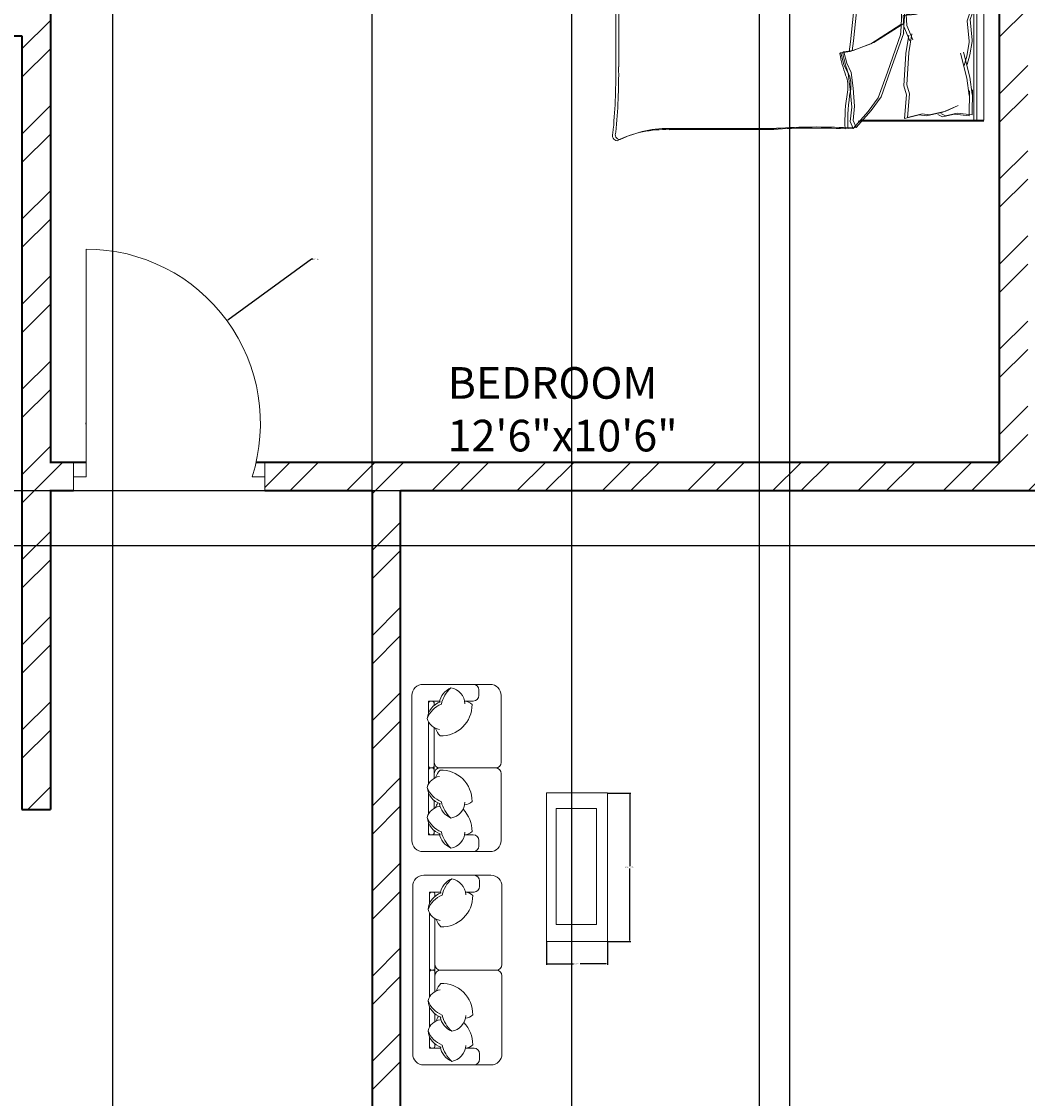
# Model space of a CAD drawing. Units: inches. Extents: x 2064 to 2782, y 1196 to 2299.
# Tile 7 of 11: x 2331 to 2490, y 1963 to 2133. Entities that reach past the tile are written whole.
import ezdxf

# ---------------------------------------------------------------- set-up
doc = ezdxf.new("R2010")
doc.units = ezdxf.units.IN
for name, color, linetype, lineweight in [('A-ANNO-DIMS', 2, 'Continuous', 18), ('A-AREA-IDEN', 7, 'Continuous', 18), ('A-DOOR', 11, 'Continuous', 18), ('A-FURN', 8, 'Continuous', 13), ('A-WALL', 7, 'Continuous', 35), ('A-WALL-PATT', 9, 'Continuous', 13)]:
    doc.layers.add(name, color=color, linetype=linetype, lineweight=lineweight)
doc.styles.get("Standard").update_dxf_attribs({"font": 'arial.ttf'})
doc.dimstyles.get("Standard").update_dxf_attribs({"dimtxt": 0.18, "dimasz": 0.18, "dimexe": 0.18, "dimexo": 0.0625, "dimgap": 0.09, "dimtad": 0, "dimtih": 1, "dimtoh": 1, "dimdec": 4, "dimzin": 0, "dimdsep": 46, "dimtxsty": 'Standard', "dimcen": 0.09, "dimadec": 0, "dimazin": 0, "dimtfac": 1, "dimtdec": 4, "dimtofl": 0, "dimtmove": 0, "dimatfit": 3, "dimfxl": 1, "dimtolj": 1, "dimtzin": 0, "dimarcsym": 0})

# ---------------------------------------------------------------- blocks, each defined once
blk = doc.blocks.new('BED-DOUBLE')
for p, q in [((2.53, 46.14), (2.53, 59.33)), ((2.53, 46.14), (2.53, 59.33)), ((2.53, 59.33), (37.35, 59.33)), ((2.53, 58.22), (37.35, 58.22)), ((2.53, 58.22), (37.35, 58.22)), ((2.7, 45.67), (2.7, 58.87)), ((2.7, 45.67), (2.7, 58.87)), ((17.88, 57.55), (18.93, 57.97)), ((17.88, 57.55), (18.93, 57.97)), ((18.93, 57.97), (19.35, 54.07)), ((18.93, 57.97), (19.35, 54.07)), ((37.35, 59.33), (37.35, 39.95)), ((37.35, 59.33), (37.35, 39.95)), ((37.52, 59.33), (37.52, 58.87)), ((37.52, 58.87), (37.52, 39.48)), ((37.52, 58.87), (37.52, 39.48)), ((2.7, 57.75), (37.52, 57.75)), ((2.7, 57.75), (37.52, 57.75)), ((2.84, 56.9), (5.96, 57.14)), ((2.84, 56.9), (5.96, 57.14)), ((2.84, 56.92), (3.26, 54.6)), ((2.84, 56.92), (3.26, 54.6)), ((3, 56.45), (3.43, 54.14)), ((3, 56.45), (3.43, 54.14)), ((3.01, 56.44), (6.13, 56.68)), ((3.01, 56.44), (6.13, 56.68)), ((5.96, 57.14), (6.04, 57.13)), ((5.96, 57.14), (6.04, 57.13)), ((6.04, 57.13), (8.82, 56.92)), ((6.04, 57.13), (8.82, 56.92)), ((6.13, 56.68), (6.2, 56.66)), ((6.13, 56.68), (6.2, 56.66)), ((6.2, 56.66), (8.99, 56.45)), ((6.2, 56.66), (8.99, 56.45)), ((8.82, 56.92), (12.82, 56.18)), ((8.82, 56.92), (12.82, 56.18)), ((8.99, 56.45), (12.99, 55.72)), ((8.99, 56.45), (12.99, 55.72)), ((10.82, 56.6), (12.3, 57.13)), ((10.82, 56.6), (12.3, 57.13)), ((10.99, 56.14), (12.46, 56.66)), ((10.99, 56.14), (12.46, 56.66)), ((12.3, 57.13), (14.4, 57.66)), ((12.3, 57.13), (14.4, 57.66)), ((12.46, 56.66), (14.57, 57.19)), ((12.46, 56.66), (14.57, 57.19)), ((14.4, 57.66), (14.64, 57.66)), ((14.4, 57.66), (14.64, 57.66)), ((14.57, 57.19), (14.8, 57.19)), ((14.57, 57.19), (14.8, 57.19)), ((14.64, 57.66), (17.88, 57.55)), ((14.64, 57.66), (17.88, 57.55)), ((14.8, 57.19), (18.04, 57.09)), ((14.8, 57.19), (18.04, 57.09)), ((18.04, 57.09), (19.1, 57.51)), ((18.04, 57.09), (19.1, 57.51)), ((19.1, 57.51), (19.52, 53.61)), ((19.1, 57.51), (19.52, 53.61)), ((20.38, 57.52), (20.2, 53.6)), ((20.38, 57.52), (20.21, 53.6)), ((20.55, 57.05), (20.37, 53.14)), ((20.55, 57.05), (20.37, 53.14)), ((21.46, 57.16), (20.38, 57.52)), ((21.46, 57.16), (20.38, 57.52)), ((21.63, 56.7), (20.55, 57.05)), ((21.63, 56.7), (20.55, 57.05)), ((24.69, 57.47), (21.46, 57.16)), ((24.69, 57.47), (21.46, 57.16)), ((24.85, 57.01), (21.63, 56.7)), ((24.85, 57.01), (21.63, 56.7)), ((24.92, 57.49), (24.69, 57.47)), ((24.92, 57.49), (24.69, 57.47)), ((25.09, 57.02), (24.85, 57.01)), ((25.09, 57.02), (24.85, 57.01)), ((27.05, 57.09), (24.92, 57.49)), ((27.05, 57.09), (24.92, 57.49)), ((27.22, 56.63), (25.09, 57.02)), ((27.22, 56.63), (25.09, 57.02)), ((30.54, 57.1), (26.59, 56.11)), ((30.54, 57.1), (26.59, 56.11)), ((30.7, 56.63), (26.75, 55.65)), ((30.7, 56.63), (26.75, 55.65)), ((28.56, 56.66), (27.05, 57.09)), ((28.56, 56.66), (27.05, 57.09)), ((28.73, 56.19), (27.22, 56.63)), ((28.73, 56.19), (27.22, 56.63)), ((33.3, 57.48), (30.54, 57.1)), ((33.3, 57.48), (30.54, 57.1)), ((33.47, 57.02), (30.7, 56.63)), ((33.47, 57.02), (30.7, 56.63)), ((36.51, 57.47), (32.57, 57.54)), ((32.57, 57.54), (33.3, 57.48)), ((36.51, 57.47), (32.57, 57.54)), ((32.57, 57.54), (33.3, 57.48)), ((36.68, 57.01), (32.74, 57.08)), ((32.74, 57.08), (33.47, 57.02)), ((36.67, 57.01), (32.74, 57.08)), ((32.74, 57.08), (33.47, 57.02)), ((36.51, 57.47), (36.23, 55.13)), ((36.51, 57.47), (36.23, 55.13)), ((36.68, 57.01), (36.4, 54.67)), ((36.67, 57.01), (36.4, 54.67)), ((3.26, 54.6), (2.94, 52.71)), ((3.26, 54.6), (2.94, 52.71)), ((3.68, 52.81), (4.42, 54.81)), ((3.68, 52.81), (4.42, 54.81)), ((35.92, 53.32), (35.06, 55.27)), ((35.92, 53.32), (35.06, 55.27)), ((36.09, 52.85), (35.23, 54.8)), ((36.09, 52.85), (35.23, 54.8)), ((36.23, 55.13), (36.67, 53.26)), ((36.23, 55.13), (36.67, 53.26)), ((36.4, 54.67), (36.83, 52.79)), ((36.4, 54.67), (36.83, 52.79)), ((3.43, 54.14), (3.11, 52.24)), ((3.43, 54.14), (3.11, 52.24)), ((3.26, 50.18), (3.68, 52.81)), ((3.26, 50.18), (3.68, 52.81)), ((3.85, 52.34), (4.58, 54.35)), ((3.85, 52.34), (4.58, 54.35)), ((19.35, 54.07), (19.77, 51.76)), ((19.35, 54.07), (19.77, 51.76)), ((19.52, 53.61), (19.94, 51.29)), ((19.52, 53.61), (19.94, 51.29)), ((20.21, 53.6), (19.93, 51.26)), ((20.2, 53.6), (19.93, 51.26)), ((20.37, 53.14), (20.1, 50.8)), ((20.37, 53.14), (20.1, 50.8)), ((36.51, 50.72), (35.92, 53.32)), ((36.51, 50.72), (35.92, 53.32)), ((36.68, 50.25), (36.09, 52.85)), ((36.67, 50.25), (36.09, 52.85)), ((36.67, 53.26), (36.29, 52.5)), ((36.67, 53.26), (36.29, 52.5)), ((2.94, 52.71), (3.36, 51.97)), ((2.94, 52.71), (3.36, 51.97)), ((3.11, 52.24), (3.53, 51.5)), ((3.11, 52.24), (3.53, 51.5)), ((3.43, 49.71), (3.85, 52.34)), ((3.43, 49.71), (3.85, 52.34)), ((19.77, 51.76), (19.77, 50.81)), ((19.77, 51.76), (19.77, 50.81)), ((19.93, 51.26), (19.99, 50.32)), ((19.93, 51.26), (19.99, 50.32)), ((19.94, 51.29), (19.94, 50.34)), ((19.94, 51.29), (19.94, 50.34)), ((36.83, 52.79), (36.46, 52.03)), ((36.83, 52.79), (36.46, 52.03)), ((3.47, 49.02), (3.26, 50.18)), ((3.47, 49.02), (3.26, 50.18)), ((3.64, 48.55), (3.43, 49.71)), ((3.64, 48.55), (3.43, 49.71)), ((19.77, 50.81), (19.35, 49.44)), ((19.77, 50.81), (19.35, 49.44)), ((19.35, 49.44), (19.35, 47.49)), ((19.35, 49.44), (19.35, 47.49)), ((19.94, 50.34), (19.52, 48.97)), ((19.94, 50.34), (19.52, 48.97)), ((19.99, 50.32), (20.49, 48.98)), ((19.99, 50.32), (20.49, 48.98)), ((20.1, 50.8), (20.15, 49.85)), ((20.1, 50.8), (20.15, 49.85)), ((20.15, 49.85), (20.66, 48.51)), ((20.15, 49.85), (20.66, 48.51)), ((36.37, 49.55), (36.51, 50.72)), ((36.37, 49.55), (36.51, 50.72)), ((36.94, 47.26), (36.37, 49.55)), ((36.94, 47.26), (36.37, 49.55)), ((36.54, 49.08), (36.68, 50.25)), ((36.54, 49.08), (36.67, 50.25)), ((3.05, 46.7), (3.47, 49.02)), ((3.05, 46.7), (3.47, 49.02)), ((3.21, 46.24), (3.64, 48.55)), ((3.21, 46.24), (3.64, 48.55)), ((4.65, 47.95), (7.59, 47.46)), ((4.65, 47.95), (7.59, 47.46)), ((17.56, 47.49), (15.27, 48.28)), ((17.56, 47.49), (15.27, 48.28)), ((17.73, 47.02), (15.44, 47.82)), ((17.73, 47.02), (15.44, 47.82)), ((19.52, 48.97), (19.52, 47.02)), ((19.52, 48.97), (19.52, 47.02)), ((20.49, 48.98), (20.62, 47.03)), ((20.49, 48.98), (20.62, 47.03)), ((20.66, 48.51), (20.78, 46.56)), ((20.66, 48.51), (20.78, 46.56)), ((22.4, 47.14), (24.64, 48.08)), ((22.4, 47.14), (24.64, 48.08)), ((23.72, 47.95), (26.66, 47.46)), ((23.72, 47.95), (26.66, 47.46)), ((37.1, 46.79), (36.54, 49.08)), ((37.1, 46.79), (36.54, 49.08)), ((6.76, 47.23), (3.05, 46.7)), ((6.76, 47.23), (3.05, 46.7)), ((6.93, 46.76), (3.21, 46.24)), ((6.93, 46.76), (3.21, 46.24)), ((4.82, 47.48), (7.75, 47)), ((4.82, 47.48), (7.75, 47)), ((7.59, 47.46), (6.76, 47.23)), ((7.59, 47.46), (6.76, 47.23)), ((7.75, 47), (6.93, 46.76)), ((7.75, 47), (6.93, 46.76)), ((7.59, 47.46), (12.69, 47.15)), ((7.59, 47.46), (12.69, 47.15)), ((7.75, 47), (12.86, 46.68)), ((7.75, 47), (12.86, 46.68)), ((12.69, 47.15), (14.12, 47.55)), ((12.69, 47.15), (14.12, 47.55)), ((12.86, 46.68), (14.29, 47.09)), ((12.86, 46.68), (14.29, 47.09)), ((14.12, 47.55), (17.86, 47.26)), ((14.12, 47.55), (17.86, 47.26)), ((14.29, 47.09), (18.03, 46.79)), ((14.29, 47.09), (18.03, 46.79)), ((19.35, 47.49), (17.56, 47.49)), ((19.35, 47.49), (17.56, 47.49)), ((19.52, 47.02), (17.73, 47.02)), ((19.52, 47.02), (17.73, 47.02)), ((20.62, 47.03), (22.4, 47.14)), ((20.62, 47.03), (22.4, 47.14)), ((20.78, 46.56), (22.57, 46.67)), ((20.78, 46.56), (22.57, 46.67)), ((22.05, 46.67), (25.1, 41.94)), ((22.05, 46.67), (25.1, 41.94)), ((22.21, 46.2), (25.26, 41.47)), ((22.21, 46.2), (25.26, 41.47)), ((22.57, 46.67), (24.81, 47.61)), ((22.57, 46.67), (24.81, 47.61)), ((29.61, 44.53), (23.54, 46.67)), ((29.61, 44.53), (23.54, 46.67)), ((29.78, 44.07), (23.7, 46.2)), ((29.78, 44.07), (23.7, 46.2)), ((23.89, 47.48), (26.83, 47)), ((23.89, 47.48), (26.83, 47)), ((26.66, 47.46), (31.77, 47.15)), ((26.66, 47.46), (31.77, 47.15)), ((26.83, 47), (31.94, 46.68)), ((26.83, 47), (31.94, 46.68)), ((31.77, 47.15), (33.2, 47.55)), ((31.77, 47.15), (33.2, 47.55)), ((31.94, 46.68), (33.36, 47.09)), ((31.94, 46.68), (33.36, 47.09)), ((33.2, 47.55), (36.94, 47.26)), ((33.2, 47.55), (36.94, 47.26)), ((33.36, 47.09), (37.1, 46.79)), ((33.36, 47.09), (37.1, 46.79)), ((33.67, 43.07), (29.61, 44.53)), ((33.67, 43.07), (29.61, 44.53)), ((33.84, 42.6), (29.78, 44.07)), ((33.84, 42.6), (29.78, 44.07)), ((35.82, 41.49), (33.67, 43.07)), ((35.82, 41.49), (33.67, 43.07)), ((35.98, 41.02), (33.84, 42.6)), ((35.98, 41.02), (33.84, 42.6)), ((25.1, 41.94), (26.34, 38.67)), ((25.1, 41.94), (26.34, 38.67)), ((25.26, 41.47), (26.51, 38.2)), ((25.26, 41.47), (26.51, 38.2)), ((38.52, 39.12), (35.82, 41.49)), ((38.52, 39.12), (35.82, 41.49)), ((38.68, 38.65), (35.98, 41.02)), ((38.68, 38.65), (35.98, 41.02)), ((26.34, 38.67), (26.56, 37.2)), ((26.34, 38.67), (26.56, 37.2)), ((26.51, 38.2), (26.73, 36.74)), ((26.51, 38.2), (26.73, 36.74)), ((26.56, 37.2), (28.37, 37.65)), ((26.56, 37.2), (28.37, 37.65)), ((28.37, 37.65), (29.84, 38.33)), ((28.37, 37.65), (29.84, 38.33)), ((28.54, 37.19), (30, 37.87)), ((28.54, 37.19), (30, 37.87)), ((29.84, 38.33), (32.32, 38.67)), ((29.84, 38.33), (32.32, 38.67)), ((30, 37.87), (32.49, 38.2)), ((30, 37.87), (32.49, 38.2)), ((32.32, 38.67), (35.14, 38.9)), ((32.32, 38.67), (35.14, 38.9)), ((32.49, 38.2), (35.31, 38.43)), ((32.49, 38.2), (35.31, 38.43)), ((35.14, 38.9), (37.4, 38.67)), ((35.14, 38.9), (37.4, 38.67)), ((35.31, 38.43), (37.56, 38.2)), ((35.31, 38.43), (37.56, 38.2)), ((37.4, 38.67), (38.52, 39.12)), ((37.4, 38.67), (38.52, 39.12)), ((37.56, 38.2), (38.68, 38.65)), ((37.56, 38.2), (38.68, 38.65)), ((38.57, 37.85), (38.52, 39.12, 2.82)), ((38.57, 37.85), (38.52, 39.12, 2.82)), ((38.74, 37.38), (38.68, 38.65, 2.82)), ((38.74, 37.38), (38.68, 38.65, 2.82)), ((26.73, 36.74), (28.54, 37.19)), ((26.73, 36.74), (28.54, 37.19)), ((10.97, 1.6), (28.91, 1.6)), ((10.97, 1.6), (28.91, 1.6)), ((11.14, 1.14), (29.07, 1.14)), ((11.14, 1.14), (29.07, 1.14))]:
    blk.add_line(p, q)
for centre, radius, start, end in [((62.04, 44.69), 60.69, 178.7218, 185.604), ((62.04, 44.69), 60.69, 178.7218, 185.604), ((15.56, -73.3), 120.19, 86.0865, 96.7821), ((15.56, -73.3), 120.19, 86.0865, 96.7821), ((15.73, -73.76), 120.19, 86.0865, 96.7821), ((15.73, -73.76), 120.19, 86.0865, 96.7821), ((62.21, 44.23), 60.69, 178.7218, 185.604), ((62.21, 44.23), 60.69, 178.7218, 185.604), ((12.94, -54.55), 94, 81.7845, 96.9006), ((12.94, -54.55), 94, 81.7845, 96.9006), ((13.1, -55.01), 94, 81.7845, 96.9006), ((13.1, -55.01), 94, 81.7845, 96.9006), ((-121.89, 36.62), 123.93, 358.4762, 1.0082), ((-121.89, 36.62), 123.93, 358.4762, 1.0082), ((-121.72, 36.16), 123.93, 358.4762, 1.0082), ((-121.72, 36.16), 123.93, 358.4762, 1.0082), ((22.7, 58.25), 21.6, 280.6617, 289.8806), ((22.7, 58.25), 21.6, 280.6617, 289.8806), ((31.87, 33.79), 4.53, 78.6608, 113.7384), ((31.87, 33.79), 4.53, 78.6608, 113.7384), ((32.04, 33.32), 4.53, 78.6608, 113.7384), ((32.04, 33.32), 4.53, 78.6608, 113.7384), ((37.39, 64.18), 26.36, 259.8763, 272.5657), ((37.39, 64.18), 26.36, 259.8763, 272.5657), ((37.56, 63.72), 26.36, 259.8763, 272.5657), ((37.56, 63.72), 26.36, 259.8763, 272.5657), ((132.79, 32.88), 94.35, 176.9791, 183.8365), ((132.79, 32.88), 94.35, 176.9791, 183.8365), ((26.69, 37.16), 0.134, 160.2464, 271.1377), ((26.69, 37.16), 0.134, 160.2464, 271.1377), ((26.86, 36.69), 0.134, 160.2464, 271.1377), ((26.86, 36.69), 0.134, 160.2464, 271.1377), ((22.86, 57.79), 21.6, 280.6617, 289.8806), ((22.86, 57.79), 21.6, 280.6617, 289.8806), ((132.95, 32.41), 94.35, 176.9791, 183.8365), ((132.95, 32.41), 94.35, 176.9791, 183.8365), ((353.21, 22.46), 351.38, 178.2277, 181.7185), ((353.21, 22.46), 351.38, 178.2277, 181.7185), ((353.38, 21.99), 351.38, 178.2277, 181.7185), ((353.38, 21.99), 351.38, 178.2277, 181.7185), ((-3284.8, 9.92), 3323.5, 0.00217, 0.28689), ((-3284.8, 9.92), 3323.5, 0.00217, 0.28689), ((-3284.64, 9.46), 3323.5, 0.00217, 0.28689), ((-3284.64, 9.46), 3323.5, 0.00217, 0.28689), ((-19.6, 12.33), 21.59, 346.0648, 358.9113), ((-19.6, 12.33), 21.59, 346.0648, 358.9113), ((-19.43, 11.87), 21.59, 346.0648, 358.9113), ((-19.43, 11.87), 21.59, 346.0648, 358.9113), ((55.48, 9.31), 16.8, 177.4714, 206.4681), ((55.48, 9.31), 16.8, 177.4714, 206.4681), ((55.65, 8.84), 16.8, 177.4714, 206.4681), ((55.65, 8.84), 16.8, 177.4714, 206.4681), ((-15.78, 8.14), 17.17, 337.9751, 356.652), ((-15.78, 8.14), 17.17, 337.9751, 356.652), ((-15.61, 7.67), 17.17, 337.9751, 356.652), ((-15.61, 7.67), 17.17, 337.9751, 356.652), ((-12.55, 76.61), 77.56, 283.3832, 287.7053), ((-12.55, 76.61), 77.56, 283.3832, 287.7053), ((-12.38, 76.14), 77.56, 283.3832, 287.7053), ((-12.38, 76.14), 77.56, 283.3832, 287.7053), ((39.64, 1.87), 0.803, 242.6588, 356.02), ((39.64, 1.87), 0.803, 242.6588, 356.02), ((0.79, 1.26), 0.793, 146.1736, 293.4781), ((0.79, 1.26), 0.793, 146.1736, 293.4781), ((0.96, 0.79), 0.793, 146.1736, 293.4781), ((0.96, 0.79), 0.793, 146.1736, 293.4781), ((15.61, -86.98), 88.71, 92.9958, 99.4091), ((15.61, -86.98), 88.71, 92.9958, 99.4091), ((15.78, -87.45), 88.71, 92.9958, 99.4091), ((15.78, -87.45), 88.71, 92.9958, 99.4091), ((29.98, -95.32), 96.92, 84.4998, 90.6351), ((29.98, -95.32), 96.92, 84.4998, 90.6351), ((30.15, -95.78), 96.92, 84.4998, 90.6351), ((30.15, -95.78), 96.92, 84.4998, 90.6351), ((39.81, 1.41), 0.803, 242.6588, 356.02), ((39.81, 1.41), 0.803, 242.6588, 356.02)]:
    blk.add_arc(centre, radius, start, end)
blk = doc.blocks.new('TABLE-COFFEE')
for points in [[(0, 23.5), (9.66, 23.5), (9.66, 0), (0, 0)], [(1.54, 21.03), (7.9, 21.03), (7.9, 2.7), (1.54, 2.7)]]:
    blk.add_lwpolyline(points, close=True)
blk = doc.blocks.new('*D20')
at = {"layer": 'A-ANNO-DIMS', "color": 0, "lineweight": -2, "transparency": 16777216}
for p, q in [((2423.4, 2011.01), (2427.04, 2011.01)), ((2426.86, 2010.83), (2426.86, 1999.45)), ((2426.86, 1987.7), (2426.86, 1999.08)), ((2423.4, 1987.52), (2427.04, 1987.52))]:
    blk.add_line(p, q, dxfattribs=at)
at = {"layer": 'A-ANNO-DIMS', "color": 0, "transparency": 16777216}
for points in [[(2426.83, 2010.83), (2426.89, 2010.83), (2426.86, 2011.01)], [(2426.83, 1987.7), (2426.89, 1987.7), (2426.86, 1987.52)]]:
    blk.add_solid(points, dxfattribs=at)
at = {"layer": 'Defpoints', "color": 0, "transparency": 16777216}
for p in [(2423.33, 2011.01), (2426.86, 2011.01), (2423.33, 1987.52)]:
    blk.add_point(p, dxfattribs=at)
at = {"layer": 'A-ANNO-DIMS', "color": 0, "transparency": 16777216, "insert": (2426.86, 1999.27), "char_height": 0.18, "attachment_point": 5}
blk.add_mtext('\\A1;TABLE 23 TYP.', dxfattribs=at)
blk = doc.blocks.new('*D21')
at = {"layer": 'A-ANNO-DIMS', "color": 0, "lineweight": -2, "transparency": 16777216}
for p, q in [((2413.68, 1987.45), (2413.68, 1983.81)), ((2423.33, 1987.45), (2423.33, 1983.81)), ((2413.86, 1983.99), (2417.99, 1983.99)), ((2423.15, 1983.99), (2419.03, 1983.99))]:
    blk.add_line(p, q, dxfattribs=at)
at = {"layer": 'A-ANNO-DIMS', "color": 0, "transparency": 16777216}
for points in [[(2413.86, 1984.02), (2413.86, 1983.96), (2413.68, 1983.99)], [(2423.15, 1984.02), (2423.15, 1983.96), (2423.33, 1983.99)]]:
    blk.add_solid(points, dxfattribs=at)
at = {"layer": 'Defpoints', "color": 0, "transparency": 16777216}
for p in [(2413.68, 1987.52), (2423.33, 1987.52), (2423.33, 1983.99)]:
    blk.add_point(p, dxfattribs=at)
at = {"layer": 'A-ANNO-DIMS', "color": 0, "transparency": 16777216, "insert": (2418.51, 1983.99), "char_height": 0.18, "attachment_point": 5}
blk.add_mtext('\\A1;10 TYP.', dxfattribs=at)
blk = doc.blocks.new('*D23')
at = {"layer": 'A-ANNO-DIMS', "color": 0, "lineweight": -2, "transparency": 16777216}
for p, q in [((2653.23, 2234.29), (2688.85, 2234.29)), ((2688.67, 2234.11), (2688.67, 1937.72)), ((2688.67, 1640.97), (2688.67, 1937.36)), ((2452.23, 1640.79), (2688.85, 1640.79))]:
    blk.add_line(p, q, dxfattribs=at)
at = {"layer": 'A-ANNO-DIMS', "color": 0, "transparency": 16777216}
for points in [[(2688.64, 2234.11), (2688.7, 2234.11), (2688.67, 2234.29)], [(2688.64, 1640.97), (2688.7, 1640.97), (2688.67, 1640.79)]]:
    blk.add_solid(points, dxfattribs=at)
at = {"layer": 'Defpoints', "color": 0, "transparency": 16777216}
for p in [(2653.17, 2234.29), (2688.67, 2234.29), (2452.17, 1640.79)]:
    blk.add_point(p, dxfattribs=at)
at = {"layer": 'A-ANNO-DIMS', "color": 0, "transparency": 16777216, "insert": (2688.67, 1937.54), "char_height": 0.18, "attachment_point": 5}
blk.add_mtext('\\A1;593.5', dxfattribs=at)
blk = doc.blocks.new('*D27')
at = {"layer": 'A-ANNO-DIMS', "color": 0, "lineweight": -2, "transparency": 16777216}
for p, q in [((2452.17, 1640.85), (2452.17, 2269.97)), ((2452.35, 2269.79), (2493.09, 2269.79)), ((2534.61, 2269.79), (2493.87, 2269.79)), ((2534.79, 1643.35), (2534.79, 2269.97))]:
    blk.add_line(p, q, dxfattribs=at)
at = {"layer": 'A-ANNO-DIMS', "color": 0, "transparency": 16777216}
for points in [[(2452.35, 2269.82), (2452.35, 2269.76), (2452.17, 2269.79)], [(2534.61, 2269.82), (2534.61, 2269.76), (2534.79, 2269.79)]]:
    blk.add_solid(points, dxfattribs=at)
at = {"layer": 'Defpoints', "color": 0, "transparency": 16777216}
for p in [(2534.79, 2269.79), (2534.79, 1643.29), (2452.17, 1640.79)]:
    blk.add_point(p, dxfattribs=at)
at = {"layer": 'A-ANNO-DIMS', "color": 0, "transparency": 16777216, "insert": (2493.48, 2269.79), "char_height": 0.18, "attachment_point": 5}
blk.add_mtext('\\A1;82.62', dxfattribs=at)
blk = doc.blocks.new('*D35')
at = {"layer": 'A-ANNO-DIMS', "color": 0, "lineweight": -2, "transparency": 16777216}
for p, q in [((2309.4, 1932.85), (2309.4, 2269.97)), ((2309.58, 2269.79), (2347.37, 2269.79)), ((2385.94, 2269.79), (2348.16, 2269.79)), ((2386.12, 1856.35), (2386.12, 2269.97))]:
    blk.add_line(p, q, dxfattribs=at)
at = {"layer": 'A-ANNO-DIMS', "color": 0, "transparency": 16777216}
for points in [[(2309.58, 2269.82), (2309.58, 2269.76), (2309.4, 2269.79)], [(2385.94, 2269.82), (2385.94, 2269.76), (2386.12, 2269.79)]]:
    blk.add_solid(points, dxfattribs=at)
at = {"layer": 'Defpoints', "color": 0, "transparency": 16777216}
for p in [(2386.12, 2269.79), (2309.4, 1932.79), (2386.12, 1856.29)]:
    blk.add_point(p, dxfattribs=at)
at = {"layer": 'A-ANNO-DIMS', "color": 0, "transparency": 16777216, "insert": (2347.76, 2269.79), "char_height": 0.18, "attachment_point": 5}
blk.add_mtext('\\A1;76.72', dxfattribs=at)
blk = doc.blocks.new('*D36')
at = {"layer": 'A-ANNO-DIMS', "color": 0, "lineweight": -2, "transparency": 16777216}
for p, q in [((2390.62, 2058.73), (2390.62, 1539.01)), ((2541.17, 2058.73), (2541.17, 1539.01)), ((2390.8, 1539.19), (2465.44, 1539.19)), ((2540.99, 1539.19), (2466.35, 1539.19))]:
    blk.add_line(p, q, dxfattribs=at)
at = {"layer": 'A-ANNO-DIMS', "color": 0, "transparency": 16777216}
for points in [[(2390.8, 1539.22), (2390.8, 1539.16), (2390.62, 1539.19)], [(2540.99, 1539.22), (2540.99, 1539.16), (2541.17, 1539.19)]]:
    blk.add_solid(points, dxfattribs=at)
at = {"layer": 'Defpoints', "color": 0, "transparency": 16777216}
for p in [(2390.62, 2058.79), (2541.17, 2058.79), (2541.17, 1539.19)]:
    blk.add_point(p, dxfattribs=at)
at = {"layer": 'A-ANNO-DIMS', "color": 0, "transparency": 16777216, "insert": (2465.9, 1539.19), "char_height": 0.18, "attachment_point": 5}
blk.add_mtext('\\A1;150.55', dxfattribs=at)
blk = doc.blocks.new('*D39')
at = {"layer": 'A-ANNO-DIMS', "color": 0, "lineweight": -2, "transparency": 16777216}
for p, q in [((2322.95, 1645.35), (2322.95, 2269.97)), ((2323.13, 2269.79), (2333.59, 2269.79)), ((2344.97, 2269.79), (2334.51, 2269.79)), ((2345.15, 1645.35), (2345.15, 2269.97))]:
    blk.add_line(p, q, dxfattribs=at)
at = {"layer": 'A-ANNO-DIMS', "color": 0, "transparency": 16777216}
for points in [[(2323.13, 2269.82), (2323.13, 2269.76), (2322.95, 2269.79)], [(2344.97, 2269.82), (2344.97, 2269.76), (2345.15, 2269.79)]]:
    blk.add_solid(points, dxfattribs=at)
at = {"layer": 'Defpoints', "color": 0, "transparency": 16777216}
for p in [(2345.15, 2269.79), (2322.95, 1645.29), (2345.15, 1645.29)]:
    blk.add_point(p, dxfattribs=at)
at = {"layer": 'A-ANNO-DIMS', "color": 0, "transparency": 16777216, "insert": (2334.05, 2269.79), "char_height": 0.18, "attachment_point": 5}
blk.add_mtext('\\A1;22.194', dxfattribs=at)
blk = doc.blocks.new('*D40')
at = {"layer": 'A-ANNO-DIMS', "color": 0, "lineweight": -2, "transparency": 16777216}
for p, q in [((2648.61, 2058.79), (2092.49, 2058.79)), ((2092.67, 2058.61), (2092.67, 2054.63)), ((2092.67, 2050.29), (2092.67, 2054.27)), ((2648.61, 2050.11), (2092.49, 2050.11))]:
    blk.add_line(p, q, dxfattribs=at)
at = {"layer": 'A-ANNO-DIMS', "color": 0, "transparency": 16777216}
for points in [[(2092.64, 2058.61), (2092.7, 2058.61), (2092.67, 2058.79)], [(2092.64, 2050.29), (2092.7, 2050.29), (2092.67, 2050.11)]]:
    blk.add_solid(points, dxfattribs=at)
at = {"layer": 'Defpoints', "color": 0, "transparency": 16777216}
for p in [(2092.67, 2058.79), (2648.67, 2058.79), (2648.67, 2050.11)]:
    blk.add_point(p, dxfattribs=at)
at = {"layer": 'A-ANNO-DIMS', "color": 0, "transparency": 16777216, "insert": (2092.67, 2054.45), "char_height": 0.18, "attachment_point": 5}
blk.add_mtext('\\A1;8.682', dxfattribs=at)
blk = doc.blocks.new('*D41')
at = {"layer": 'A-ANNO-DIMS', "color": 0, "lineweight": -2, "transparency": 16777216}
for p, q in [((2417.67, 2229.73), (2417.67, 1539.01)), ((2447.29, 2229.73), (2447.29, 1539.01)), ((2417.85, 1539.19), (2432.08, 1539.19)), ((2447.11, 1539.19), (2432.87, 1539.19))]:
    blk.add_line(p, q, dxfattribs=at)
at = {"layer": 'A-ANNO-DIMS', "color": 0, "transparency": 16777216}
for points in [[(2417.85, 1539.22), (2417.85, 1539.16), (2417.67, 1539.19)], [(2447.11, 1539.22), (2447.11, 1539.16), (2447.29, 1539.19)]]:
    blk.add_solid(points, dxfattribs=at)
at = {"layer": 'Defpoints', "color": 0, "transparency": 16777216}
for p in [(2417.67, 2229.79), (2447.29, 2229.79), (2447.29, 1539.19)]:
    blk.add_point(p, dxfattribs=at)
at = {"layer": 'A-ANNO-DIMS', "color": 0, "transparency": 16777216, "insert": (2432.48, 1539.19), "char_height": 0.18, "attachment_point": 5}
blk.add_mtext('\\A1;29.62', dxfattribs=at)
blk = doc.blocks.new('*D46')
at = {"layer": 'A-ANNO-DIMS', "color": 0, "lineweight": -2, "transparency": 16777216}
for p, q in [((2376.56, 2095.46), (2363.34, 2085.82)), ((2376.74, 2095.46), (2376.56, 2095.46)), ((2340.83, 2069.48), (2341.01, 2069.48)), ((2340.92, 2069.39), (2340.92, 2069.57))]:
    blk.add_line(p, q, dxfattribs=at)
at = {"layer": 'A-ANNO-DIMS', "color": 0, "transparency": 16777216}
blk.add_solid([(2363.32, 2085.84), (2363.36, 2085.8), (2363.2, 2085.71)], dxfattribs=at)
at = {"layer": 'Defpoints', "color": 0, "transparency": 16777216}
for p in [(2363.2, 2085.71), (2340.92, 2069.48)]:
    blk.add_point(p, dxfattribs=at)
at = {"layer": 'A-ANNO-DIMS', "color": 0, "transparency": 16777216, "insert": (2377.29, 2095.46), "char_height": 0.18, "attachment_point": 5}
blk.add_mtext('\\A1;R27.565', dxfattribs=at)

msp = doc.modelspace()

# ---------------------------------------------------------------- hatches: boundary and pattern name
at = {"layer": 'A-WALL-PATT'}
h = msp.add_hatch(dxfattribs=at)
h.set_pattern_fill('ANSI32', color=256)
h.paths.add_polyline_path([(2489.7688, 2189.2917), (2574.5454, 2189.2917), (2574.5454, 2191.5417), (2574.5454, 2193.7917), (2570.6691, 2193.7917), (2570.6691, 2197.3052), (2568.4191, 2197.3052), (2566.1691, 2197.3052), (2566.1691, 2193.7917), (2494.1691, 2193.7917), (2494.1691, 2229.7917), (2523.2441, 2229.7917), (2523.2441, 2234.2917), (2471.2886, 2234.2917), (2471.2886, 2229.7917), (2489.6691, 2229.7917), (2489.6691, 2193.7917), (2417.6691, 2193.7917), (2417.6691, 2197.0632), (2415.4191, 2197.0632), (2413.1691, 2197.0632), (2413.1691, 2193.7917), (2406.8865, 2193.7917), (2406.8865, 2189.2917), (2485.2688, 2189.2917), (2485.2688, 2063.2917), (2369.1629, 2063.2917), (2369.1629, 2058.7917), (2386.1222, 2058.7917), (2386.1222, 1856.2917), (2382.1576, 1856.2917), (2382.1576, 1851.7917), (2394.9764, 1851.7917), (2394.9764, 1854.0417), (2394.9764, 1856.2917), (2390.6222, 1856.2917), (2390.6222, 2058.7917), (2485.2688, 2058.7917), (2493.762, 2058.7917), (2493.762, 2061.0417), (2493.762, 2063.2917), (2489.7688, 2063.2917)])
h.paths.add_polyline_path([(2447.2886, 2234.2917), (2413.1691, 2234.2917), (2413.1691, 2217.3799), (2417.6691, 2217.3799), (2417.6691, 2229.7917), (2447.2886, 2229.7917)], flags=17)
h.paths.add_polyline_path([(2570.6691, 2234.2917), (2547.2441, 2234.2917), (2547.2441, 2229.7917), (2566.1691, 2229.7917), (2566.1691, 2216.5615), (2570.6691, 2216.5615)], flags=17)
h.paths.add_polyline_path([(2653.1691, 2189.2917), (2653.1691, 2193.7917), (2640.8843, 2193.7917), (2640.8843, 2189.2917), (2648.6691, 2189.2917), (2648.6691, 2162.7138), (2653.1691, 2162.7138)])
h.paths.add_polyline_path([(2653.1691, 2102.7138), (2648.6691, 2102.7138), (2648.6691, 2063.2917), (2526.7281, 2063.2917), (2526.7281, 2058.7917), (2541.1691, 2058.7917), (2541.1691, 1993.2917), (2545.6691, 1993.2917), (2545.6691, 1997.7917), (2545.6691, 2058.7917), (2648.6691, 2058.7917), (2648.6691, 2050.1099), (2653.1691, 2050.1099)])
h.paths.add_polyline_path([(2600.6691, 1856.2917), (2493.4607, 1856.2917), (2493.4607, 1851.7917), (2596.1691, 1851.7917), (2596.1691, 1695.7917), (2594.0816, 1695.7917), (2594.0816, 1691.2917), (2614.7905, 1691.2917), (2614.7905, 1645.2917), (2536.7905, 1645.2917), (2536.7905, 1691.2917), (2539.332, 1691.2917), (2539.332, 1693.5417), (2539.332, 1695.7917), (2452.1691, 1695.7917), (2452.1691, 1851.7917), (2456.0775, 1851.7917), (2456.0775, 1856.2917), (2427.1536, 1856.2917), (2427.1536, 1851.7917), (2447.6691, 1851.7917), (2447.6691, 1695.7917), (2447.6691, 1645.2917), (2405.1469, 1645.2917), (2405.1469, 1640.7917), (2452.1691, 1640.7917), (2452.1691, 1645.2917), (2452.1691, 1691.2917), (2534.7905, 1691.2917), (2534.7905, 1645.2917), (2534.7905, 1643.2917), (2614.7905, 1643.2917), (2616.7905, 1643.2917), (2616.7905, 1691.2917), (2622.4029, 1691.2917), (2622.4029, 1693.7143), (2622.4029, 1695.7917), (2600.6691, 1695.7917), (2600.6691, 1779.7917), (2648.6691, 1779.7917), (2648.6691, 1695.7917), (2646.4029, 1695.7917), (2646.4029, 1691.2917), (2653.1691, 1691.2917), (2653.1691, 1906.3508), (2648.6691, 1906.3508), (2648.6691, 1856.2917), (2648.6691, 1784.2917), (2600.6691, 1784.2917)])
h.paths.add_polyline_path([(2322.9532, 1819.5181), (2320.7032, 1819.5181), (2318.4532, 1819.5181), (2318.4532, 1695.7917), (2242.7664, 1695.7917), (2242.7664, 1691.2917), (2318.4532, 1691.2917), (2318.4532, 1640.7917), (2322.9532, 1640.7917), (2345.1469, 1640.7917), (2345.1469, 1643.0417), (2345.1469, 1645.2917), (2322.9532, 1645.2917), (2322.9532, 1691.2917), (2322.9532, 1695.7917)])
h.paths.add_polyline_path([(2166.1825, 1691.2917), (2164.1825, 1691.2917), (2164.1825, 1643.2917), (2166.1825, 1643.2917), (2246.1825, 1643.2917), (2246.1825, 1645.2917), (2246.1825, 1691.2917), (2244.1825, 1691.2917), (2244.1825, 1645.2917), (2166.1825, 1645.2917)])
h.paths.add_polyline_path([(2309.404, 1932.7917), (2204.1691, 1932.7917), (2204.1691, 1960.0962), (2199.6691, 1960.0962), (2199.6691, 1932.7917), (2132.6691, 1932.7917), (2132.6691, 1951.0737), (2128.1691, 1951.0737), (2128.1691, 1910.0412), (2132.6691, 1910.0412), (2132.6691, 1928.2917), (2304.904, 1928.2917), (2304.904, 1856.2917), (2304.904, 1851.7917), (2318.4532, 1851.7917), (2318.4532, 1848.8308), (2322.9532, 1848.8308), (2322.9532, 1851.7917), (2347.7631, 1851.7917), (2347.7631, 1856.2917), (2309.404, 1856.2917)])
h.paths.add_polyline_path([(2132.6691, 2044.9092), (2130.4191, 2044.9092), (2128.1691, 2044.9092), (2128.1691, 1987.0737), (2132.6691, 1987.0737), (2132.6691, 2004.7917), (2199.6691, 2004.7917), (2204.1691, 2004.7917), (2204.1691, 2009.2917), (2132.6691, 2009.2917)])
h.paths.add_polyline_path([(2186.6691, 2195.9329), (2184.4191, 2195.9329), (2184.4191, 2195.8929), (2182.1691, 2195.9329), (2182.1691, 2193.7917), (2128.1691, 2193.7917), (2128.1691, 2181.4967), (2132.6691, 2181.4967), (2132.6691, 2182.7769), (2132.6691, 2189.2917), (2182.1691, 2189.2917), (2182.1691, 2135.2917), (2179.804, 2135.2917), (2179.804, 2130.7917), (2190.215, 2130.7917), (2190.215, 2133.0417), (2190.215, 2135.2917), (2186.6691, 2135.2917)])
h.paths.add_polyline_path([(2340.0628, 2189.2917), (2340.0628, 2191.5417), (2340.0628, 2193.7917), (2335.1691, 2193.7917), (2335.1691, 2234.2917), (2280.6746, 2234.2917), (2280.6746, 2229.7917), (2330.6691, 2229.7917), (2330.6691, 2193.7917), (2330.6691, 2135.2917), (2218.6309, 2135.2917), (2218.6309, 2130.7917), (2330.7688, 2130.7917), (2330.7688, 2008.4023), (2335.2688, 2008.4023), (2335.2688, 2058.7917), (2338.9208, 2058.7917), (2338.9208, 2061.0417), (2338.9208, 2063.2917), (2335.2688, 2063.2917), (2335.2688, 2189.2917)])
h.paths.add_polyline_path([(2220.6746, 2234.2917), (2182.1691, 2234.2917), (2182.1691, 2227.4187), (2186.6691, 2227.4187), (2186.6691, 2229.7917), (2220.6746, 2229.7917), (2220.6746, 2232.0417)])
h.paths.add_polyline_path([(2158.8146, 2135.2917), (2132.6691, 2135.2917), (2132.6691, 2157.4967), (2128.1691, 2157.4967), (2128.1691, 2104.9092), (2132.6691, 2104.9092), (2132.6691, 2130.7917), (2158.8146, 2130.7917), (2158.8146, 2133.0417)])
h.paths.add_polyline_path([(2396.0464, 2062.2045), (2434.8868, 2062.2045), (2434.8868, 2080.8619), (2396.0464, 2080.8619)], flags=24)
h.paths.add_polyline_path([(2196.1396, 1653.3449), (2232.023, 1653.3449), (2232.023, 1672.0022), (2196.1396, 1672.0022)], flags=25)

# ---------------------------------------------------------------- linework, layer by layer
at = {"layer": 'A-DOOR'}
for p, q in [((2340.9208, 2061.0417), (2340.9208, 2097.0417)), ((2338.9208, 2063.2917), (2338.9208, 2058.7917)), ((2369.1629, 2063.2917), (2369.1629, 2058.7917)), ((2369.1629, 2058.7917), (2369.1629, 2063.2917)), ((2338.9208, 2058.7917), (2338.9208, 2061.0417)), ((2338.9208, 2061.0417), (2340.9208, 2061.0417)), ((2369.1629, 2061.0417), (2367.1629, 2061.0417))]:
    msp.add_line(p, q, dxfattribs=at)
msp.add_arc((2340.9208, 2069.4772), 27.5645, 342.180047, 90, dxfattribs=at)
at = {"layer": 'A-FURN', "ltscale": 0.03}
for points in [[(2406.5361, 2015.852, -0.41421356), (2405.6541, 2014.97, -0.41421356), (2406.5361, 2014.088), (2406.5361, 2003.504, -0.41421356), (2404.7721, 2001.7401), (2394.1881, 2001.7401, -0.41421356), (2392.4241, 2003.504), (2392.4241, 2026.436, -0.41421356), (2394.1881, 2028.2), (2404.7721, 2028.2, -0.41421356), (2406.5361, 2026.436), (2406.5361, 2015.852, -0.41421356), (2405.6541, 2014.97, -0.41421356), (2406.5361, 2014.088)], [(2406.6546, 1983.8792, -0.41421356), (2405.7726, 1982.9972, -0.41421356), (2406.6546, 1982.1152), (2406.6546, 1969.7672, -0.41421356), (2404.8906, 1968.0032), (2394.3066, 1968.0032, -0.41421356), (2392.5426, 1969.7672), (2392.5426, 1996.2271, -0.41421356), (2394.3066, 1997.9911), (2404.8906, 1997.9911, -0.41421356), (2406.6546, 1996.2271), (2406.6546, 1983.8792, -0.41421356), (2405.7726, 1982.9972, -0.41421356), (2406.6546, 1982.1152)]]:
    msp.add_lwpolyline(points, format="xyb", dxfattribs=at)
at = {"layer": 'A-FURN'}
for points in [[(2398.5898, 2027.6386, 0.14772988), (2397.074, 2025.0608, 0.21334276), (2394.8508, 2022.7863, 0.17866181)], [(2400.813, 2025.1114, 0.35677236), (2398.5898, 2027.6386, 0.24954205), (2396.7577, 2025.3487, -9.61688035)], [(2402.1261, 2028.2, -0.41421356), (2403.0081, 2027.318), (2403.0081, 2026.436, -0.41421356), (2402.1261, 2025.554), (2400.7596, 2025.554)], [(2395.9521, 2024.8809), (2395.9521, 2025.2012, 0.41421356), (2395.5993, 2025.554), (2395.4229, 2025.554, 0.41421356), (2395.0701, 2025.2012)], [(2400.7592, 2025.5559, -0.16554063), (2401.9245, 2025.0103, -0.42598917), (2396.8719, 2020.0568, -0.12152332), (2396.1754, 2021.2327, 7.11546429)], [(2396.9532, 2025.4169, 0.30666349), (2394.8508, 2022.7863, 0.30632997), (2396.7708, 2021.0677, -0.87284716)], [(2395.0701, 2025.2012), (2395.0701, 2023.6985, 0.41421356)], [(2395.0701, 2022.2312), (2395.0701, 2015.3228, 0.41421356), (2395.4229, 2014.97), (2395.5993, 2014.97, 0.41421356), (2395.9521, 2015.3228), (2395.9521, 2021.3431, 0.41421356)], [(2395.9521, 2015.852, 0.41421356), (2396.8341, 2014.97)], [(2395.9521, 2015.852, 0.41421356), (2396.8341, 2014.97), (2405.6541, 2014.97, 0.41421356)], [(2396.9532, 2009.2744, -0.30666349), (2394.8508, 2011.905, -0.30632997), (2396.7708, 2013.6236, 0.87284716)], [(2395.0701, 2012.4601), (2395.0701, 2014.6172, -0.41421356), (2395.4229, 2014.97), (2395.5993, 2014.97, -0.41421356), (2395.9521, 2014.6172), (2395.9521, 2013.3482, -0.41421356)], [(2395.9521, 2014.088, -0.41421356), (2396.8341, 2014.97)], [(2395.9521, 2014.088, -0.41421356), (2396.8341, 2014.97), (2405.6541, 2014.97, -0.41421356)], [(2400.7592, 2009.1354, 0.16554063), (2401.9245, 2009.681, 0.42598917), (2396.8719, 2014.6345, 0.12152332), (2396.1754, 2013.4587, -7.11546429)], [(2398.5898, 2007.0527, -0.14772988), (2397.074, 2009.6305, -0.21334276), (2394.8508, 2011.905, -0.17866181)], [(2395.0701, 2007.7088), (2395.0701, 2010.9928, -0.41421356)], [(2396.9532, 2004.5231, -0.30666349), (2394.8508, 2007.1538, -0.30632997), (2396.7708, 2008.8723, 0.87284716)], [(2395.9521, 2009.8104), (2395.9521, 2008.597, -0.41421356)], [(2396.5203, 2009.4468, 0.07186538), (2396.1754, 2008.7074, -7.11546429)], [(2400.813, 2009.58, -0.35677236), (2398.5898, 2007.0527, -0.24954205), (2396.7577, 2009.3426, 9.61688035)], [(2400.7592, 2004.3841, 0.16554063), (2401.9245, 2004.9298, 0.20023115), (2400.5052, 2008.431, 0.12152332)], [(2398.5898, 2002.3014, -0.14772988), (2397.074, 2004.8792, -0.21334276), (2394.8508, 2007.1538, -0.17866181)], [(2395.0701, 2004.7388), (2395.0701, 2006.2415, -0.41421356)], [(2395.0701, 2006.2415), (2395.0701, 2004.386), (2396.8035, 2004.386, -0.41421356)], [(2395.9521, 2005.0591), (2395.9521, 2004.7388, -0.41421356), (2395.5993, 2004.386), (2395.4229, 2004.386, -0.41421356), (2395.0701, 2004.7388)], [(2400.813, 2004.8287, -0.35677236), (2398.5898, 2002.3014, -0.24954205), (2396.7577, 2004.5913, 9.61688035)], [(2400.7596, 2004.386), (2402.1261, 2004.386, -0.41421356), (2403.0081, 2003.504), (2403.0081, 2002.6221, -0.41421356), (2402.1261, 2001.7401)], [(2398.7083, 1997.4298, 0.14772988), (2397.1925, 1994.852, 0.21334276), (2394.9693, 1992.5774, 0.17866181)], [(2400.9314, 1994.9025, 0.35677236), (2398.7083, 1997.4298, 0.24954205), (2396.8762, 1995.1398, -9.61688035)], [(2402.2446, 1997.9911, -0.41421356), (2403.1266, 1997.1091), (2403.1266, 1996.2271, -0.41421356), (2402.2446, 1995.3451), (2400.8781, 1995.3451)], [(2397.0717, 1995.2081, 0.30666349), (2394.9693, 1992.5774, 0.30632997), (2396.8893, 1990.8589, -0.87284716)], [(2396.0706, 1994.6721), (2396.0706, 1994.9923, 0.41421356), (2395.7178, 1995.3451), (2395.5414, 1995.3451, 0.41421356), (2395.1886, 1994.9923)], [(2395.1886, 1994.9923), (2395.1886, 1993.4896, 0.41421356)], [(2400.8777, 1995.347, -0.16554063), (2402.043, 1994.8014, -0.42598917), (2396.9904, 1989.8479, -0.12152332), (2396.2939, 1991.0238, 7.11546429)], [(2395.1886, 1992.0223), (2395.1886, 1983.35, 0.41421356), (2395.5414, 1982.9972), (2395.7178, 1982.9972, 0.41421356), (2396.0706, 1983.35), (2396.0706, 1991.1342, 0.41421356)], [(2395.1886, 1978.7233), (2395.1886, 1982.6444, -0.41421356), (2395.5414, 1982.9972), (2395.7178, 1982.9972, -0.41421356), (2396.0706, 1982.6444), (2396.0706, 1979.6114, -0.41421356)], [(2396.0706, 1983.8792, 0.41421356), (2396.9526, 1982.9972)], [(2396.0706, 1983.8792, 0.41421356), (2396.9526, 1982.9972), (2405.7726, 1982.9972, 0.41421356)], [(2396.0706, 1982.1152, -0.41421356), (2396.9526, 1982.9972)], [(2396.0706, 1982.1152, -0.41421356), (2396.9526, 1982.9972), (2405.7726, 1982.9972, -0.41421356)], [(2397.0717, 1975.5375, -0.30666349), (2394.9693, 1978.1682, -0.30632997), (2396.8893, 1979.8868, 0.87284716)], [(2400.8777, 1975.3986, 0.16554063), (2402.043, 1975.9442, 0.42598917), (2396.9904, 1980.8977, 0.12152332), (2396.2939, 1979.7218, -7.11546429)], [(2398.7083, 1973.3158, -0.14772988), (2397.1925, 1975.8937, -0.21334276), (2394.9693, 1978.1682, -0.17866181)], [(2395.1886, 1973.972), (2395.1886, 1977.256, -0.41421356)], [(2396.0706, 1976.0736), (2396.0706, 1974.8601, -0.41421356)], [(2397.0717, 1970.7862, -0.30666349), (2394.9693, 1973.4169, -0.30632997), (2396.8893, 1975.1355, 0.87284716)], [(2396.6388, 1975.71, 0.07186538), (2396.2939, 1974.9705, -7.11546429)], [(2400.9314, 1975.8431, -0.35677236), (2398.7083, 1973.3158, -0.24954205), (2396.8762, 1975.6058, 9.61688035)], [(2400.8777, 1970.6473, 0.16554063), (2402.043, 1971.1929, 0.20023115), (2400.6237, 1974.6941, 0.12152332)], [(2398.7083, 1968.5645, -0.14772988), (2397.1925, 1971.1424, -0.21334276), (2394.9693, 1973.4169, -0.17866181)], [(2395.1886, 1972.5047), (2395.1886, 1970.6492), (2396.922, 1970.6492, -0.41421356)], [(2395.1886, 1971.002), (2395.1886, 1972.5047, -0.41421356)], [(2396.0706, 1971.3223), (2396.0706, 1971.002, -0.41421356), (2395.7178, 1970.6492), (2395.5414, 1970.6492, -0.41421356), (2395.1886, 1971.002)], [(2400.9314, 1971.0918, -0.35677236), (2398.7083, 1968.5645, -0.24954205), (2396.8762, 1970.8545, 9.61688035)], [(2400.8781, 1970.6492), (2402.2446, 1970.6492, -0.41421356), (2403.1266, 1969.7672), (2403.1266, 1968.8852, -0.41421356), (2402.2446, 1968.0032)]]:
    msp.add_lwpolyline(points, format="xyb", dxfattribs=at)
for points in [[(2396.8035, 2025.554), (2395.0701, 2025.554), (2395.0701, 2023.6985)], [(2395.0701, 2022.2312), (2395.0701, 2012.4601)], [(2395.0701, 2010.9928), (2395.0701, 2007.7088)], [(2396.922, 1995.3451), (2395.1886, 1995.3451), (2395.1886, 1993.4896)], [(2395.1886, 1992.0223), (2395.1886, 1978.7233)], [(2395.1886, 1977.256), (2395.1886, 1973.972)]]:
    msp.add_lwpolyline(points, dxfattribs=at)
for points in [[(2395.0701, 2015.3228), (2395.0701, 2014.6172, -0.41421356), (2395.4229, 2014.97), (2395.5993, 2014.97, -0.41421356), (2395.9521, 2014.6172), (2395.9521, 2015.3228, -0.41421356), (2395.5993, 2014.97), (2395.4229, 2014.97, -0.41421356)], [(2395.1886, 1983.35), (2395.1886, 1982.6444, -0.41421356), (2395.5414, 1982.9972), (2395.7178, 1982.9972, -0.41421356), (2396.0706, 1982.6444), (2396.0706, 1983.35, -0.41421356), (2395.7178, 1982.9972), (2395.5414, 1982.9972, -0.41421356)]]:
    msp.add_lwpolyline(points, format="xyb", close=True, dxfattribs=at)
at = {"layer": 'A-WALL'}
for p, q in [((2335.2688, 2189.2917), (2335.2688, 2063.2917)), ((2485.2688, 2189.2917), (2485.2688, 2063.2917)), ((2218.6309, 2130.7917), (2330.7688, 2130.7917)), ((2330.7688, 2130.7917), (2330.7688, 2008.4023)), ((2340.9208, 2063.2917), (2335.1691, 2063.2917)), ((2485.2688, 2063.2917), (2367.7824, 2063.2917)), ((2338.9208, 2058.7917), (2335.1691, 2058.7917)), ((2335.2688, 2058.7917), (2335.2688, 2008.4023)), ((2386.1222, 2058.7917), (2369.1629, 2058.7917)), ((2386.1222, 2058.7917), (2386.1222, 1856.2917)), ((2485.2688, 2058.7917), (2390.6222, 2058.7917)), ((2390.6222, 1856.2917), (2390.6222, 2058.7917)), ((2493.762, 2058.7917), (2485.2688, 2058.7917)), ((2330.7688, 2008.4023), (2335.2688, 2008.4023))]:
    msp.add_line(p, q, dxfattribs=at)

# ---------------------------------------------------------------- block references
at = {"layer": 'A-FURN', "rotation": 269.9999998331855}
msp.add_blockref('BED-DOUBLE', (2423.5043, 2154.8008), dxfattribs=at)
at = {"layer": 'A-FURN'}
msp.add_blockref('TABLE-COFFEE', (2413.6761, 1987.516), dxfattribs=at)

# ---------------------------------------------------------------- texts
at = {"layer": 'A-AREA-IDEN', "insert": (2398.057, 2078.3772), "char_height": 5, "attachment_point": 1}
msp.add_mtext_dynamic_manual_height_columns('BEDROOM\\P12\'6"x10\'6"', width=179.028955, gutter_width=12.5, heights=[0], dxfattribs=at)

# ---------------------------------------------------------------- dimensions: what is measured, and where the dimension line sits
at = {"layer": 'A-ANNO-DIMS'}
for base, p1, p2, override, picture, middle in [((2386.1222, 2269.7917), (2309.404, 1932.7917), (2386.1222, 1856.2917), {"dimdec": 2, "dimlfac": 1, "dimrnd": 0, "dimzin": 0, "dimdsep": 46, "dimlunit": 2}, '*D35', (2347.7631, 2269.7917)), ((2345.1469, 2269.7917), (2322.9532, 1645.2917), (2345.1469, 1645.2917), {"dimdec": 3, "dimlfac": 1, "dimrnd": 0, "dimzin": 0, "dimdsep": 46, "dimlunit": 2}, '*D39', (2334.0501, 2269.7917)), ((2534.7905, 2269.7917), (2452.1691, 1640.7917), (2534.7905, 1643.2917), {"dimdec": 2, "dimlfac": 1, "dimrnd": 0, "dimzin": 0, "dimdsep": 46, "dimlunit": 2}, '*D27', (2493.4798, 2269.7917)), ((2447.2886, 1539.1896), (2417.6691, 2229.7917), (2447.2886, 2229.7917), {"dimdec": 2, "dimlfac": 1, "dimrnd": 0, "dimzin": 0, "dimdsep": 46, "dimlunit": 2}, '*D41', (2432.4788, 1539.1896)), ((2541.1691, 1539.1896), (2390.6222, 2058.7917), (2541.1691, 2058.7917), {"dimdec": 2, "dimlfac": 1, "dimrnd": 0, "dimzin": 0, "dimdsep": 46, "dimlunit": 2}, '*D36', (2465.8957, 1539.1896))]:
    dim = msp.add_linear_dim(base=base, p1=p1, p2=p2, dimstyle='Standard', override=override, dxfattribs=at)
    dim.commit()
    dim.dimension.update_dxf_attribs({"geometry": picture, "text_midpoint": middle})
for base, p1, p2, override, picture, middle in [((2688.6691, 2234.2917), (2452.1691, 1640.7917), (2653.1691, 2234.2917), {"dimdec": 1, "dimlfac": 1, "dimrnd": 0, "dimzin": 0, "dimdsep": 46, "dimlunit": 2}, '*D23', (2688.6691, 1937.5417)), ((2092.6691, 2058.7917), (2648.6691, 2050.1099), (2648.6691, 2058.7917), {"dimdec": 3, "dimlfac": 1, "dimrnd": 0, "dimzin": 0, "dimdsep": 46, "dimlunit": 2}, '*D40', (2092.6691, 2054.4508))]:
    dim = msp.add_linear_dim(base=base, p1=p1, p2=p2, angle=90, dimstyle='Standard', override=override, dxfattribs=at)
    dim.commit()
    dim.dimension.update_dxf_attribs({"geometry": picture, "text_midpoint": middle})
dim = msp.add_radius_dim(center=(2340.92082, 2069.47716), mpoint=(2363.19541, 2085.7143), dimstyle='Standard', override={"dimdec": 3, "dimlfac": 1, "dimrnd": 0, "dimzin": 0, "dimdsep": 46, "dimlunit": 2}, dxfattribs=at)
dim.commit()
dim.dimension.update_dxf_attribs({"geometry": '*D46', "text_midpoint": (2377.29061, 2095.45659), "dimtype": 164})
dim = msp.add_linear_dim(base=(2426.8595, 2011.0149), p1=(2423.3347, 1987.516), p2=(2423.3347, 2011.0149), angle=90, text='TABLE <> TYP.', dimstyle='Standard', override={"dimdec": 0, "dimlfac": 1, "dimrnd": 0, "dimzin": 0, "dimdsep": 46, "dimlunit": 2}, dxfattribs=at)
dim.commit()
dim.dimension.update_dxf_attribs({"geometry": '*D20', "text_midpoint": (2426.8595, 1999.2655)})
dim = msp.add_linear_dim(base=(2423.3347, 1983.9911), p1=(2413.6761, 1987.516), p2=(2423.3347, 1987.516), text='<> TYP.', dimstyle='Standard', override={"dimdec": 0, "dimlfac": 1, "dimrnd": 0, "dimzin": 0, "dimdsep": 46, "dimlunit": 2}, dxfattribs=at)
dim.commit()
dim.dimension.update_dxf_attribs({"geometry": '*D21', "text_midpoint": (2418.5054, 1983.9911)})

doc.saveas('drawing.dxf')
